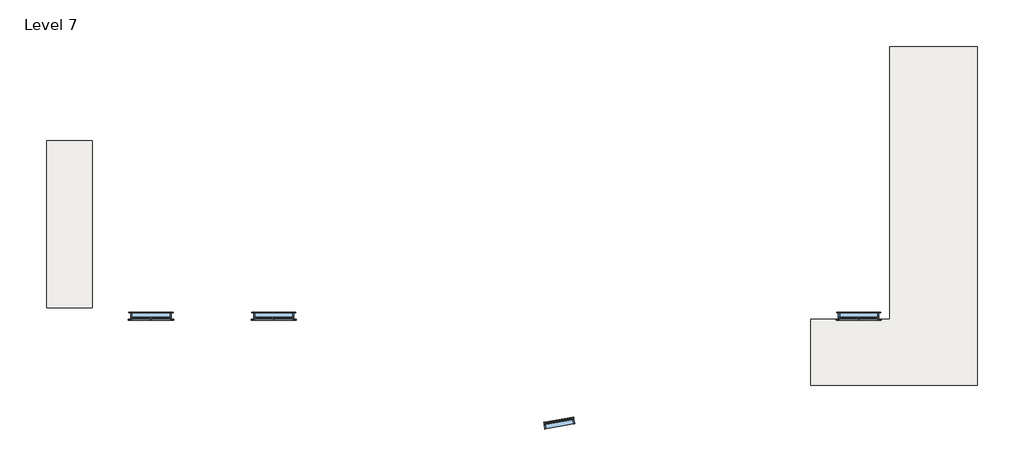
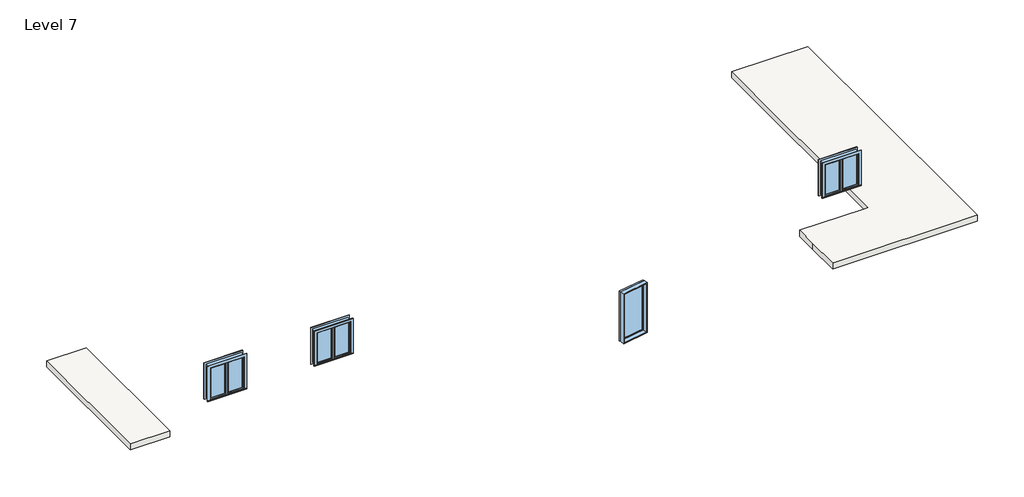
# One storey: 4 windows, 3 slabs.
"""IFC4 building model written with IfcOpenShell, lengths in millimetres."""

from ifc_helpers import new_model, si_unit, frame, origin, place, context, project, spatial, polyline, outline, extrude, transform, mapped, element, save
from components import window_0862ab64, window_9a779fa2

model = new_model("IFC4")

# Units and contexts
model_context = context("Model", 3, world=origin())
ifc_project = project(units=[si_unit("LENGTHUNIT", "METRE", prefix="MILLI")], contexts=[model_context])

# Site, building, storey
site = spatial("IfcSite", under=ifc_project)
building = spatial("IfcBuilding", under=site)
storey = spatial("IfcBuildingStorey", under=building, Name="Level 7", Elevation=9829.8)

# Slabs
placement = place(None, origin())
element("IfcSlab", 1, ObjectType="9\"", at=placement, inside=storey, context=model_context, shape_type="SweptSolid", body=[
    extrude(outline(polyline([(-17979.5505427, -8690.0239591), (-16607.9505427, -8690.0239591), (-16607.9505427, -13719.2239591), (-17979.5505427, -13719.2239591), (-17979.5505427, -8690.0239591)])), frame((0.0, 0.0, 9601.2), z_axis=(0.0, 0.0, 1.0), x_axis=(1.0, 0.0, 0.0)), (0.0, 0.0, 1.0), 228.6),
])
element("IfcSlab", 2, ObjectType="9\"", at=placement, inside=storey, context=model_context, shape_type="SweptSolid", body=[
    extrude(outline(polyline([(-17979.5505427, -8690.0239591), (-16607.9505427, -8690.0239591), (-16607.9505427, -13719.2239591), (-17979.5505427, -13719.2239591), (-17979.5505427, -8690.0239591)])), frame((0.0, 0.0, 9601.2), z_axis=(0.0, 0.0, 1.0), x_axis=(1.0, 0.0, 0.0)), (0.0, 0.0, 1.0), 228.6),
])
element("IfcSlab", 3, ObjectType="9\"", at=placement, inside=storey, context=model_context, shape_type="SweptSolid", body=[
    extrude(outline(polyline([(5058.2494573, -14840.0808221), (5058.2494573, -14078.0808221), (7242.6494573, -14078.0808221), (7445.8494573, -14078.0808221), (7445.8494573, -5848.4808221), (10087.4494573, -5848.4808221), (10087.4494573, -14840.0808221), (10087.4494573, -16059.2808221), (5058.2494573, -16059.2808221), (5058.2494573, -14840.0808221)])), frame((0.0, 0.0, 9601.2), z_axis=(0.0, 0.0, 1.0), x_axis=(1.0, 0.0, 0.0)), (0.0, 0.0, 1.0), 228.6),
])

# Windows
window_shape = window_0862ab64(model_context)
element("IfcWindow", 4, ObjectType="Casement Dbl with Trim : 48\" x 48\"", at=placement, inside=storey, context=model_context, shape_type="MappedRepresentation", body=[
    mapped(window_shape, transform((-11129.6382271, -13957.4308221, 9829.8), x_axis=(-1.0, 0.0, 0.0), y_axis=(0.0, -1.0, 0.0), z_axis=(0.0, 0.0, 1.0))),
])
element("IfcWindow", 5, ObjectType="Casement Dbl with Trim : 48\" x 48\"", at=placement, inside=storey, context=model_context, shape_type="MappedRepresentation", body=[
    mapped(window_shape, transform((-14829.9505427, -13957.4308221, 9829.8), x_axis=(-1.0, 0.0, 0.0), y_axis=(0.0, -1.0, 0.0), z_axis=(0.0, 0.0, 1.0))),
])
element("IfcWindow", 6, ObjectType="Casement Dbl with Trim : 48\" x 48\"", at=placement, inside=storey, context=model_context, shape_type="MappedRepresentation", body=[
    mapped(window_shape, transform((6506.0494573, -13957.4308221, 9829.8), x_axis=(-1.0, 0.0, 0.0), y_axis=(0.0, -1.0, 0.0), z_axis=(0.0, 0.0, 1.0))),
])
window_2_shape = window_9a779fa2(model_context)
element("IfcWindow", 7, ObjectType="Fixed : 36\" x 72\"", at=placement, inside=storey, context=model_context, shape_type="MappedRepresentation", body=[
    mapped(window_2_shape, transform((-2486.4769786, -17194.6292958, 10165.0447876), x_axis=(0.9848787521632385, 0.1732450389978952, 0.0), y_axis=(-0.1732450389978952, 0.9848787521632385, 0.0), z_axis=(0.0, 0.0, 1.0))),
])

save(model, "model.ifc")

# Revit data of these elements
# Type "9\""
#   Assembly Code = "B1010"
#   Function = 0
#   Layers, outside or top first: 0' - 9" no material (function 1)
# Type "Casement Dbl with Trim : 48\" x 48\""
#   Type Mark = "10"
#   Construction Type Id = "GSP4R"
#   Assembly Code = "B2020100"
#   Analytic Construction = "1/8 in Pilkington single glazing"
#   Visual Light Transmittance = 0.9
#   Solar Heat Gain Coefficient = 0.78
#   Heat Transfer Coefficient (U) = 0.6496 BTU/(h·ft²·°F)
#   Height = 4' - 0"
#   Default Sill Height = 3' - 0"
#   Trim Projection - Ext. = 0' - 0 1/2"
#   Trim Projection - Int. = 0' - 0 3/4"
#   Trim Width - Exterior = 0' - 3 1/2"
#   Trim Width - Interior = 0' - 3 1/2"
#   Width = 4' - 0"
#   Window Inset = 0' - 0 3/4"
#   Define Thermal Properties by = 1
#   Glass Pane Material = Glass
#   Sash Material = Sash
#   Trim Exterior Material = Trim
#   Trim Interior Material = Trim
#   Wall Closure = (empty or 0)
# Type "Fixed : 36\" x 72\""
#   Type Mark = "9"
#   Construction Type Id = "GSP4R"
#   Assembly Code = "B2020100"
#   Analytic Construction = "1/8 in Pilkington single glazing"
#   Visual Light Transmittance = 0.9
#   Solar Heat Gain Coefficient = 0.78
#   Heat Transfer Coefficient (U) = 0.6496 BTU/(h·ft²·°F)
#   Height = 6' - 0"
#   Default Sill Height = 1' - 0"
#   Width = 3' - 0"
#   Window Inset = 0' - 0 3/4"
#   Define Thermal Properties by = 1
#   Glass Pane Material = Glass
#   Sash Material = Sash
#   Wall Closure = (empty or 0)
# Elements 1, 2 (IfcSlab, "9\"")
#   built-in parameter 1001955 = 3.14159 (stored number, unit not read)
#   Height Offset From Level = 0' - 0"
#   Phase Created = New Construction
#   Materials on its faces: "Default Floor"
# Element 3 (IfcSlab, "9\"")
#   built-in parameter 1001955 = -1.5708 (stored number, unit not read)
#   Height Offset From Level = 0' - 0"
#   Phase Created = New Construction
#   Materials on its faces: "Default Floor"
# Element 4 (IfcWindow, "Casement Dbl with Trim : 48\" x 48\"")
#   Mark = "41"
#   Phase Created = New Construction
#   Materials on its faces: "Sash", "Trim", "Glass"
# Element 5 (IfcWindow, "Casement Dbl with Trim : 48\" x 48\"")
#   Mark = "42"
#   Phase Created = New Construction
#   Materials on its faces: "Sash", "Trim", "Glass"
# Element 6 (IfcWindow, "Casement Dbl with Trim : 48\" x 48\"")
#   Mark = "58"
#   Phase Created = New Construction
#   Materials on its faces: "Sash", "Trim", "Glass"
# Element 7 (IfcWindow, "Fixed : 36\" x 72\"")
#   Mark = "13"
#   Phase Created = New Construction
#   Materials on its faces: "Sash", "Glass"
# Materials
#   "Glass": class "Glass", colour RGB 0 128 192, transparency 0.75, Description = "Soda Lime Glass", Cost = 0
#   "Sash": class "Wood", colour RGB 224 178 126, transparency 0
#   "Trim": class "Wood", colour RGB 224 178 126, transparency 0
#   "Default Floor": colour RGB 128 128 128, transparency 0
